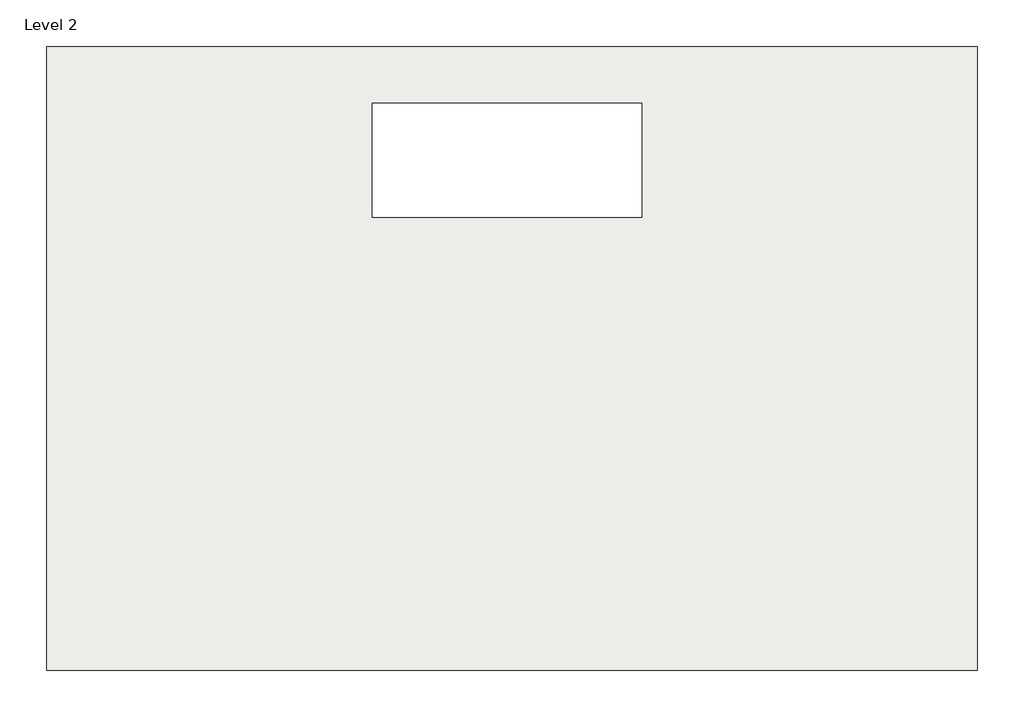
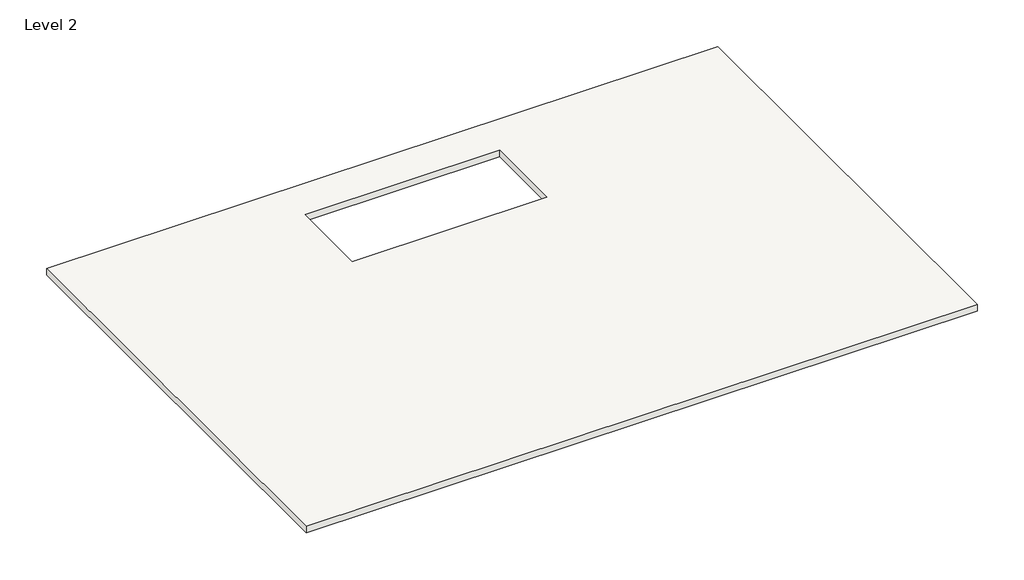
# One storey, incomplete: 1 roof.
"""IFC4 building model written with IfcOpenShell, lengths in millimetres."""

from ifc_helpers import new_model, si_unit, frame, origin, place, context, project, spatial, polyline, outline, extrude, element, save

model = new_model("IFC4")

# Units and contexts
model_context = context("Model", 3, world=origin())
ifc_project = project(units=[si_unit("LENGTHUNIT", "METRE", prefix="MILLI")], contexts=[model_context])

# Site, building, storey
site = spatial("IfcSite", under=ifc_project)
building = spatial("IfcBuilding", under=site)
storey = spatial("IfcBuildingStorey", under=building, Name="Level 2", Elevation=3048.0)

# Roof
placement = place(None, origin())
element("IfcRoof", 1, ObjectType="Generic - 12\"", at=placement, inside=storey, context=model_context, shape_type="SweptSolid", body=[
    extrude(outline(polyline([(6019.2953358, 7335.1167606), (6019.2953358, -2418.4832394), (-8534.9046642, -2418.4832394), (-8534.9046642, 7335.1167606), (6019.2953358, 7335.1167606)]), holes=[polyline([(774.1953358, 6446.1167606), (-3442.2046642, 6446.1167606), (-3442.2046642, 4668.1167606), (774.1953358, 4668.1167606), (774.1953358, 6446.1167606)])]), frame((0.0, 0.0, 3048.0), z_axis=(0.0, 0.0, 1.0), x_axis=(1.0, 0.0, 0.0)), (0.0, 0.0, 1.0), 152.4),
])

save(model, "model.ifc")

# Revit data of these elements
# Type "Generic - 12\""
#   Assembly Code = "B1020"
#   Layers, outside or top first: 0' - 6" no material (function 1)
# Element 1 (IfcRoof, "Generic - 12\"")
#   built-in parameter 1001705 = 10.5 (stored number, unit not read)
#   built-in parameter 1001710 = 33615
#   Phase Created = New Construction
#   Materials on its faces: "Default Roof"
# Materials
#   "Default Roof": colour RGB 88 101 114, transparency 0, Cost = 0
